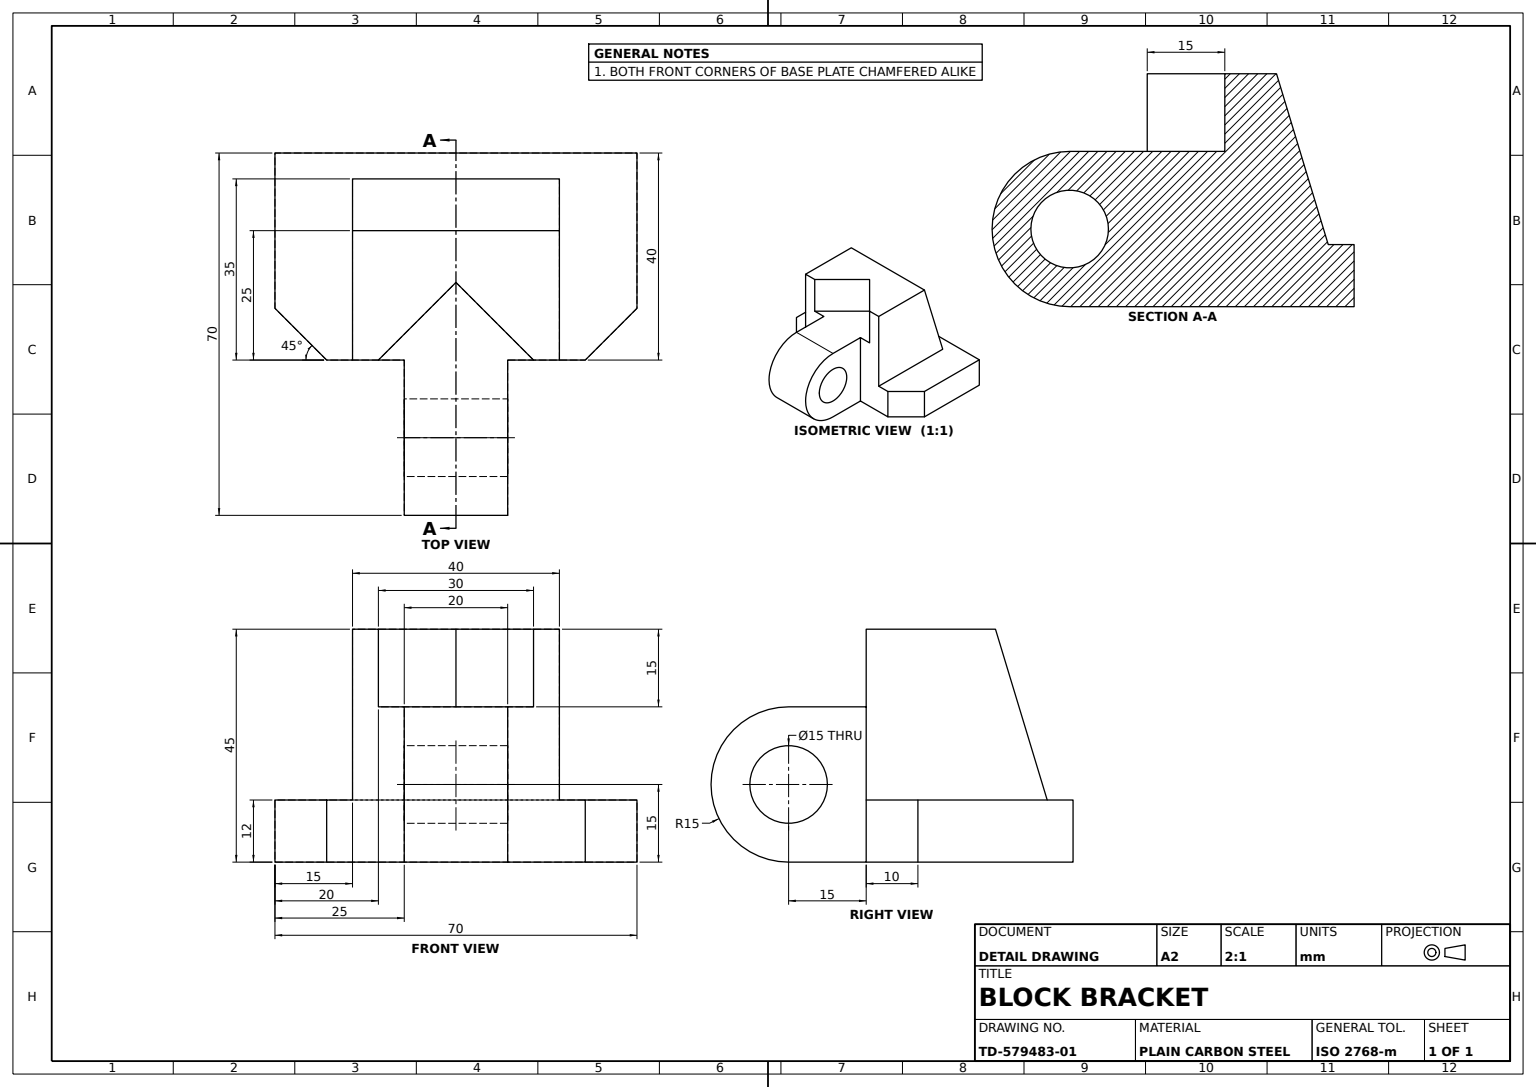
from build123d import *

# Parameters (mm, degrees)
BASE_PLATE_DEPTH        = 12
JOURNAL_BOSS_SKETCH_R   = 7.5
JOURNAL_BOSS_DEPTH      = 10
CRADLE_SLOT_30X15_DEPTH = 15


with BuildPart() as part:
    # Base Plate Sketch → Base Plate (new body)
    with BuildSketch(Plane(origin=(0, 0, 0), x_dir=(1, 0, 0), z_dir=(0, 1, 0))):
        Polygon((0, 0), (-35, 0), (-35, -30), (-25, -40), (25, -40), (35, -30), (35, 0), align=None)
    extrude(amount=BASE_PLATE_DEPTH)

    # Pedestal Top Profile → Tapered Pedestal section 0
    with BuildSketch(Plane(origin=(0, 45, 0), x_dir=(1, 0, 0), z_dir=(0, 1, 0))):
        with BuildLine():
            Line((-20, -40), (20, -40))
            Line((20, -40), (20, -15))
            Line((20, -15), (-20, -15))
            Line((-20, -15), (-20, -40))
        make_face()
    # Pedestal Bottom Profile → Tapered Pedestal section 1
    with BuildSketch(Plane(origin=(0, 12, 0), x_dir=(1, 0, 0), z_dir=(0, 1, 0))):
        with BuildLine():
            Line((-20, -40), (-20, -5))
            Line((-20, -5), (20, -5))
            Line((20, -5), (20, -40))
            Line((20, -40), (-20, -40))
        make_face()
    loft()

    # Journal Boss Sketch → Journal Boss (add, symmetric)
    with BuildSketch(Plane(origin=(0, 0, 0), x_dir=(0, 0, -1), z_dir=(1, 0, 0))):
        with BuildLine():
            Line((-40, 30), (-55, 30))
            ThreePointArc((-55, 30), (-70, 15), (-55, 0))
            Line((-55, 0), (-40, 0))
            Line((-40, 0), (-40, 30))
        make_face()
        with Locations((-55, 15)):
            Circle(JOURNAL_BOSS_SKETCH_R, mode=Mode.SUBTRACT)
    extrude(amount=JOURNAL_BOSS_DEPTH, both=True)

    # Cradle Slot Sketch → Cradle Slot 30x15 (cut)
    with BuildSketch(Plane(origin=(0, 45, 0), x_dir=(1, 0, 0), z_dir=(0, 1, 0))):
        Polygon((-15, -40), (0, -25), (15, -40), align=None)
    extrude(amount=-CRADLE_SLOT_30X15_DEPTH, mode=Mode.SUBTRACT)


solid = part.part
